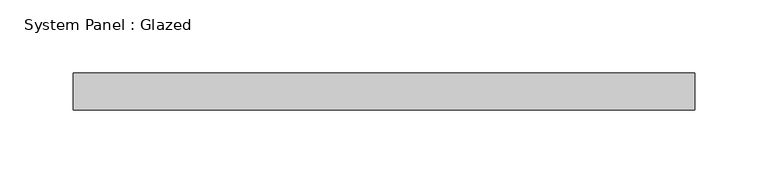
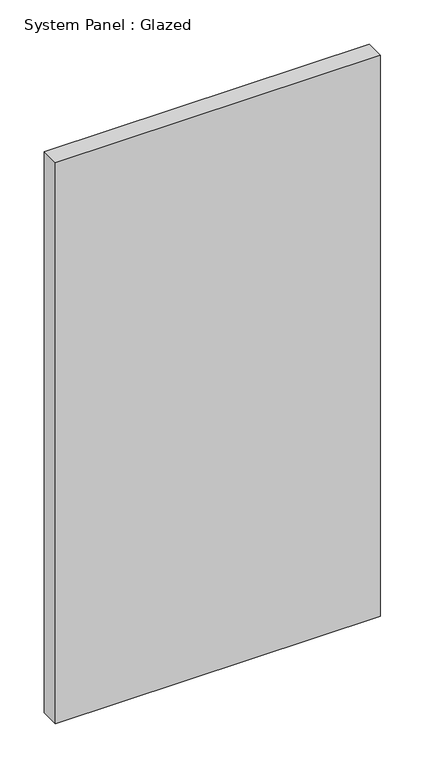
"""IFC4 building model written with IfcOpenShell, lengths in millimetres: plate geometry, System Panel : Glazed."""

from ifc_helpers import new_model, si_unit, origin, origin_with_axes, place, context, project, spatial, polyline, outline, extrude, source, transform, mapped, element, save


def system_panel_glazed_79b80f84(model_context):
    return source(origin(), model_context, "Body", "SweptSolid", [
        extrude(outline(polyline([(212.725, 19.05), (-212.725, 19.05), (-212.725, 44.45), (212.725, 44.45), (212.725, 19.05)])), origin_with_axes(), (0.0, 0.0, 1.0), 776.0351947),
    ])


if __name__ == "__main__":
    model = new_model("IFC4")
    model_context = context("Model", 3, world=origin())
    ifc_project = project(units=[si_unit("LENGTHUNIT", "METRE", prefix="MILLI")], contexts=[model_context])
    site = spatial("IfcSite", under=ifc_project)
    building = spatial("IfcBuilding", under=site)
    placement = place(None, origin())
    system_panel_glazed_shape = system_panel_glazed_79b80f84(model_context)
    element("IfcPlate", 1, ObjectType="System Panel : Glazed", at=placement, inside=building, context=model_context, shape_type="MappedRepresentation", body=[
        mapped(system_panel_glazed_shape, transform((0.0, 0.0, 0.0), x_axis=(1.0, 0.0, 0.0), y_axis=(0.0, 1.0, 0.0), z_axis=(0.0, 0.0, 1.0))),
    ])
    save(model, "model.ifc")

# Revit data of these elements
# Type "System Panel : Glazed"
#   Construction Type Id = "GSP4R"
#   Analytic Construction = "1/8 in Pilkington single glazing"
#   Visual Light Transmittance = 0.9
#   Solar Heat Gain Coefficient = 0.86
#   Heat Transfer Coefficient (U) = 1.18115 BTU/(h·ft²·°F)
#   Define Thermal Properties by = 1
# Element 1 (IfcPlate, "System Panel : Glazed")
#   Materials on its faces: "Glass"
# Materials
#   "Glass": class "Glass", colour RGB 0 128 192, transparency 0.75, Description = "Soda Lime Glass", Cost = 0
